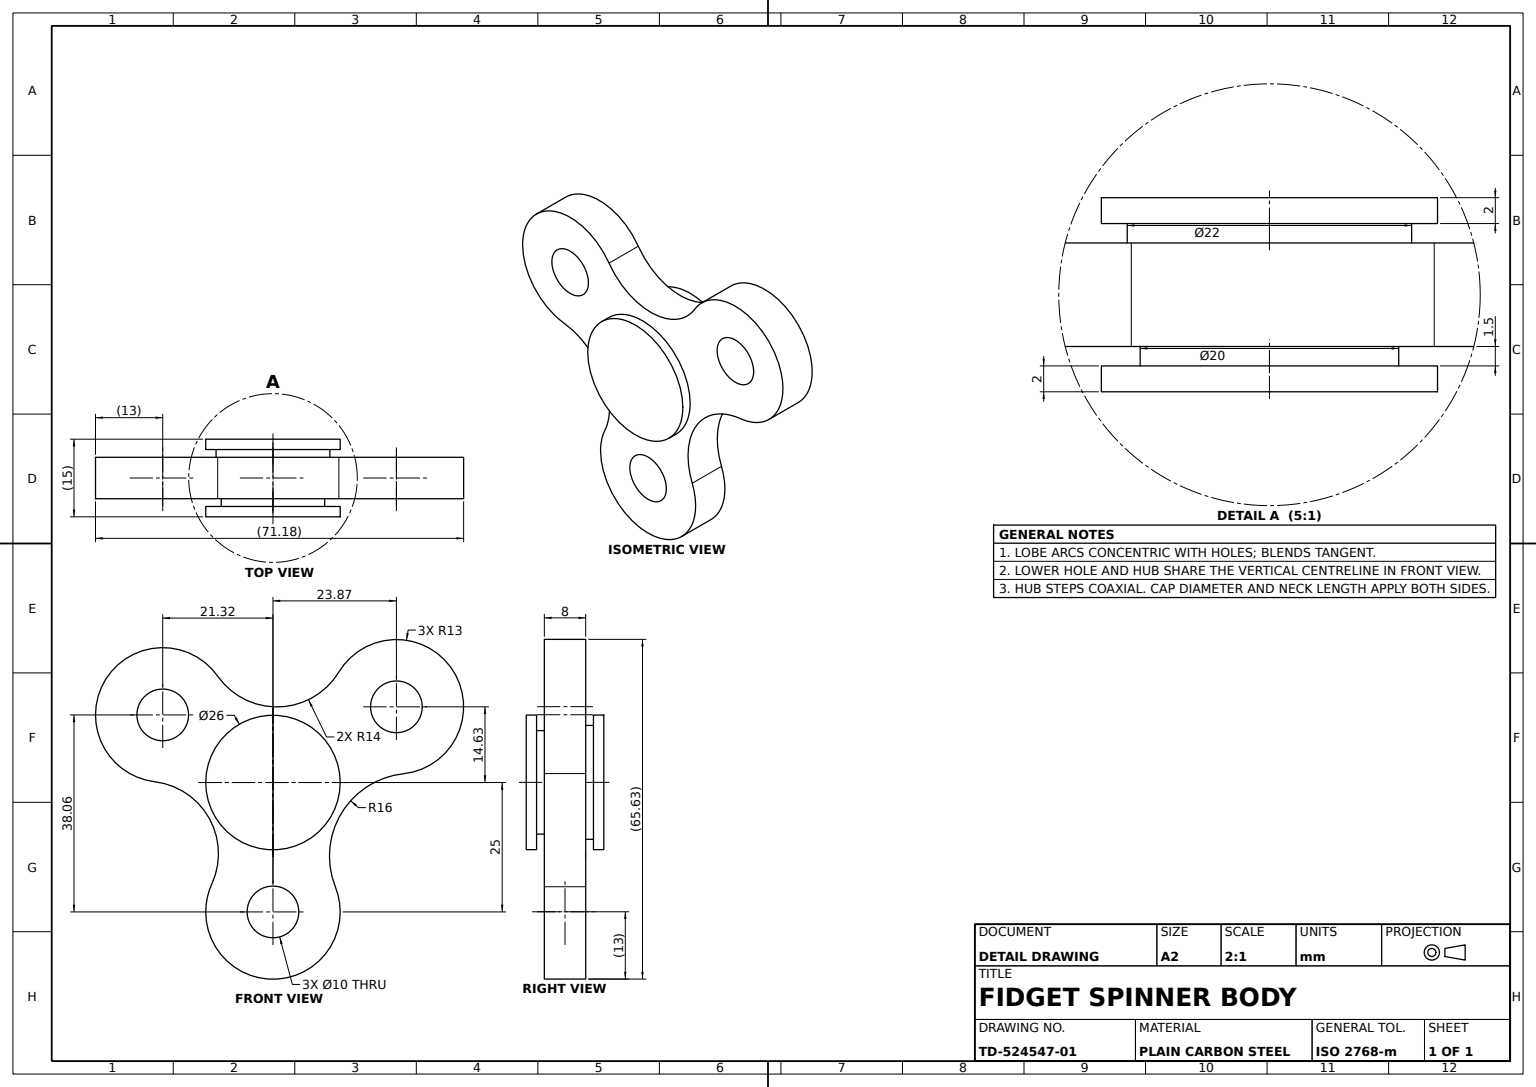
SolidWorks part; units mm, degrees
material "Plain Carbon Steel"
ref_plane "Front Plane" through (0, 0, 0) normal (0, 0, 1) x (1, 0, 0)
ref_plane "Top Plane" through (0, 0, 0) normal (0, 1, 0) x (1, 0, 0)
ref_plane "Right Plane" through (0, 0, 0) normal (1, 0, 0) x (0, 0, -1)
sketch "Spinner Body Sketch" plane through (0, 0, 0) normal (0, 0, 1) x (1, 0, 0)
  line L0 (0, 0) -> (0, -25)
  line L1 (0, 0) -> (23.8663, 14.6253)
  line L2 (0, 0) -> (-21.316, 13.0625)
  arc A0 (-11.8165, -19.5805) -> (12.0673, -20.1647) centre (0, -25) ccw
  arc A1 (25.2349, 1.6975) -> (12.7433, 21.3543) centre (23.8663, 14.6253) ccw
  arc A2 (-10.6845, 20.5439) -> (-22.8692, 0.1556) centre (-21.316, 13.0625) ccw
  arc A3 (-10.6845, 20.5439) -> (12.7433, 21.3543) centre (0.7647, 28.6009) ccw
  arc A4 (-22.8692, 0.1556) -> (-11.8165, -19.5805) centre (-24.5419, -13.7441) cw
  arc A5 (12.0673, -20.1647) -> (25.2349, 1.6975) centre (26.9194, -14.2135) cw
  dimension "D1" = 25
  dimension "D2" = 26
  dimension "D4" = 26
  dimension "D5" = 16
  dimension "D8" = 26
  dimension "D9" = 14
  dimension "D10" = 14
  dimension "D11" = 23.8663
  dimension "D3" = 31.5
  dimension "D6" = 31.5
  dimension "D7" = 25
extrude "Spinner Body" add sketch "Spinner Body Sketch" along normal blind 8
sketch "Hub Boss Ø10 Sketch" plane through (0, 0, 8) normal (0, 0, 1) x (1, 0, 0)
  circle A0 centre (0, 0) radius 10
  dimension "D1" = 10
extrude "Hub Boss Ø10" add sketch "Hub Boss Ø10 Sketch" along normal blind 1.5
sketch "Hub Boss Ø11 Sketch" plane through (0, 0, 0) normal (0, 0, -1) x (-1, 0, 0)
  circle A0 centre (0, 0) radius 11
  dimension "D1" = 11
extrude "Hub Boss Ø11" add sketch "Hub Boss Ø11 Sketch" along normal blind 1.5
sketch "Hub Cap Ø13 on Ø11 Boss Sketch" plane through (0, 0, -1.5) normal (0, 0, -1) x (-1, 0, 0)
  circle A0 centre (0, 0) radius 13
  dimension "D1" = 13
extrude "Hub Cap Ø13 on Ø11 Boss" add sketch "Hub Cap Ø13 on Ø11 Boss Sketch" along normal blind 2
sketch "Hub Cap Ø13 on Ø10 Boss Sketch" plane through (0, 0, 9.5) normal (0, 0, 1) x (1, 0, 0)
  circle A0 centre (0, 0) radius 13
  dimension "D1" = 13
extrude "Hub Cap Ø13 on Ø10 Boss" add sketch "Hub Cap Ø13 on Ø10 Boss Sketch" along normal blind 2
sketch "Lobe Holes 3xØ10 Sketch" plane through (0, 0, 0) normal (0, 0, -1) x (-1, 0, 0)
  circle A0 centre (-23.8663, 14.6253) radius 10
  circle A1 centre (21.316, 13.0625) radius 10
  circle A2 centre (0, -25) radius 10
  dimension "D1" = 10
  dimension "D2" = 10
  dimension "D3" = 10
extrude "Lobe Holes 3xØ10" cut sketch "Lobe Holes 3xØ10 Sketch" against normal blind 8
sketch "Lobe Rings 3xØ10-Ø9 Sketch" plane through (0, 0, 0) normal (0, 0, -1) x (-1, 0, 0)
  circle A0 centre (-23.8663, 14.6253) radius 9
  circle A1 centre (21.316, 13.0625) radius 9
  circle A2 centre (0, -25) radius 9
  circle A3 centre (-23.8663, 14.6253) radius 10
  circle A4 centre (21.316, 13.0625) radius 10
  circle A5 centre (0, -25) radius 10
  dimension "D1" = 9
  dimension "D2" = 9
  dimension "D3" = 9
  dimension "D4" = 10
  dimension "D5" = 10
  dimension "D6" = 10
extrude "Lobe Rings 3xØ10-Ø9" add sketch "Lobe Rings 3xØ10-Ø9 Sketch" against normal blind 8
sketch "Lobe Rings 3xØ9-Ø6 Sketch" plane through (0, 0, 0) normal (0, 0, -1) x (-1, 0, 0)
  circle A0 centre (-23.8663, 14.6253) radius 6
  circle A1 centre (-23.8663, 14.6253) radius 9
  circle A2 centre (21.316, 13.0625) radius 9
  circle A3 centre (21.316, 13.0625) radius 6
  circle A4 centre (0, -25) radius 9
  circle A5 centre (0, -25) radius 6
  dimension "D1" = 6
  dimension "D2" = 9
  dimension "D3" = 9
  dimension "D4" = 6
  dimension "D5" = 9
  dimension "D6" = 6
extrude "Lobe Rings 3xØ9-Ø6" add sketch "Lobe Rings 3xØ9-Ø6 Sketch" against normal blind 8
sketch "Lobe Rings 3xØ6-Ø5 Sketch" plane through (0, 0, 0) normal (0, 0, -1) x (-1, 0, 0)
  circle A0 centre (-23.8663, 14.6253) radius 5
  circle A1 centre (-23.8663, 14.6253) radius 6
  circle A2 centre (21.316, 13.0625) radius 6
  circle A3 centre (21.316, 13.0625) radius 5
  circle A4 centre (0, -25) radius 6
  circle A5 centre (0, -25) radius 5
  dimension "D1" = 5
  dimension "D2" = 6
  dimension "D3" = 6
  dimension "D4" = 5
  dimension "D5" = 6
  dimension "D6" = 5
extrude "Lobe Rings 3xØ6-Ø5" add sketch "Lobe Rings 3xØ6-Ø5 Sketch" against normal blind 8
